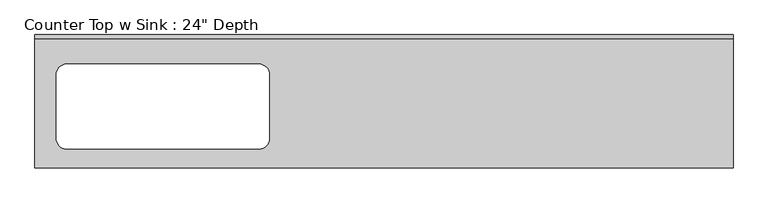
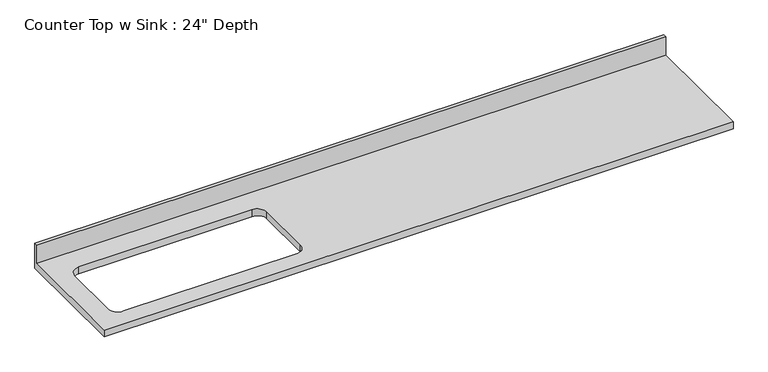
"""IFC4 building model written with IfcOpenShell, lengths in millimetres: furniture geometry."""

from ifc_helpers import new_model, si_unit, frame, origin, place, context, project, spatial, polyline, circle_curve, source, transform, mapped, element, save
from ifc_brep_helpers import plane_surface, revolved_surface, advanced_brep


def furniture_c9b163cf(model_context):
    return source(origin(), model_context, "Body", "AdvancedBrep", [
        advanced_brep(
        [(-1200.4622951, -635.0, 914.4), (2126.9377049, -635.0, 914.4), (2126.9377049, -19.05, 914.4), (-1200.4622951, -19.05, 914.4), (-1048.0622951, -139.7, 914.4), (-133.6622951, -139.7, 914.4), (-82.8622951, -190.5, 914.4), (-82.8622951, -495.3, 914.4), (-133.6622951, -546.1, 914.4), (-1048.0622951, -546.1, 914.4), (-1098.8622951, -495.3, 914.4), (-1098.8622951, -190.5, 914.4), (2126.9377049, 0.0, 876.3), (2126.9377049, -635.0, 876.3), (-1200.4622951, -635.0, 876.3), (-1200.4622951, 0.0, 876.3), (-133.6622951, -139.7, 876.3), (-1048.0622951, -139.7, 876.3), (-1098.8622951, -190.5, 876.3), (-1098.8622951, -495.3, 876.3), (-1048.0622951, -546.1, 876.3), (-133.6622951, -546.1, 876.3), (-82.8622951, -495.3, 876.3), (-82.8622951, -190.5, 876.3), (-1200.4622951, 0.0, 1016.0), (2126.9377049, 0.0, 1016.0), (-1200.4622951, -19.05, 1016.0), (2126.9377049, -19.05, 1016.0)],
        [
            (0, 1),
            (1, 2),
            (2, 3),
            (3, 0),
            (4, 5),
            (5, 6, circle_curve(frame((-133.6622951, -190.5, 914.4), z_axis=(0.0, 0.0, -1.0), x_axis=(1.0, 0.0, 0.0)), 50.8)),
            (6, 7),
            (7, 8, circle_curve(frame((-133.6622951, -495.3, 914.4), z_axis=(0.0, 0.0, -1.0), x_axis=(1.0, 0.0, 0.0)), 50.8)),
            (8, 9),
            (9, 10, circle_curve(frame((-1048.0622951, -495.3, 914.4), z_axis=(0.0, 0.0, -1.0), x_axis=(1.0, 0.0, 0.0)), 50.8)),
            (10, 11),
            (11, 4, circle_curve(frame((-1048.0622951, -190.5, 914.4), z_axis=(0.0, 0.0, -1.0), x_axis=(1.0, 0.0, 0.0)), 50.8)),
            (12, 13),
            (13, 14),
            (14, 15),
            (15, 12),
            (16, 17),
            (17, 18, circle_curve(frame((-1048.0622951, -190.5, 876.3), z_axis=(0.0, 0.0, 1.0), x_axis=(1.0, 0.0, 0.0)), 50.8)),
            (18, 19),
            (19, 20, circle_curve(frame((-1048.0622951, -495.3, 876.3), z_axis=(0.0, 0.0, 1.0), x_axis=(1.0, 0.0, 0.0)), 50.8)),
            (20, 21),
            (21, 22, circle_curve(frame((-133.6622951, -495.3, 876.3), z_axis=(0.0, 0.0, 1.0), x_axis=(1.0, 0.0, 0.0)), 50.8)),
            (22, 23),
            (23, 16, circle_curve(frame((-133.6622951, -190.5, 876.3), z_axis=(0.0, 0.0, 1.0), x_axis=(1.0, 0.0, 0.0)), 50.8)),
            (15, 24),
            (24, 25),
            (25, 12),
            (14, 0),
            (3, 26),
            (26, 24),
            (13, 1),
            (25, 27),
            (27, 2),
            (26, 27),
            (4, 17),
            (16, 5),
            (11, 18),
            (10, 19),
            (9, 20),
            (8, 21),
            (7, 22),
            (6, 23),
        ],
        [
            plane_surface(frame((-1200.4622951, 0.0, 914.4), z_axis=(0.0, 0.0, 1.0), x_axis=(-1.0, 0.0, 0.0))),
            plane_surface(frame((-1200.4622951, 0.0, 876.3), z_axis=(0.0, 0.0, -1.0), x_axis=(1.0, 0.0, 0.0))),
            plane_surface(frame((2126.9377049, 0.0, 914.4), z_axis=(0.0, 1.0, 0.0), x_axis=(0.0, 0.0, -1.0))),
            plane_surface(frame((-1200.4622951, 0.0, 914.4), z_axis=(-1.0, 0.0, 0.0), x_axis=(0.0, 0.0, -1.0))),
            plane_surface(frame((-1200.4622951, -635.0, 914.4), z_axis=(0.0, -1.0, 0.0), x_axis=(0.0, 0.0, -1.0))),
            plane_surface(frame((2126.9377049, -635.0, 914.4), z_axis=(1.0, 0.0, 0.0), x_axis=(0.0, 0.0, -1.0))),
            plane_surface(frame((-1200.4622951, 0.0, 1016.0), z_axis=(0.0, 0.0, 1.0), x_axis=(0.0, -1.0, 0.0))),
            plane_surface(frame((-1200.4622951, -19.05, 1016.0), z_axis=(0.0, -1.0, 0.0), x_axis=(0.0, 0.0, -1.0))),
            plane_surface(frame((-133.6622951, -139.7, 914.4), z_axis=(0.0, -1.0, 0.0), x_axis=(0.0, 0.0, -1.0))),
            revolved_surface(polyline([(-997.2622951000001, -190.5, 914.4), (-997.2622951000001, -190.5, 876.3)]), (-1048.0622951, -190.5, 876.3), (0.0, 0.0, 1.0)),
            plane_surface(frame((-1098.8622951, -190.5, 914.4), z_axis=(1.0, 0.0, 0.0), x_axis=(0.0, 0.0, -1.0))),
            revolved_surface(polyline([(-997.2622951000001, -495.3, 914.4), (-997.2622951000001, -495.3, 876.3)]), (-1048.0622951, -495.3, 876.3), (0.0, 0.0, 1.0)),
            plane_surface(frame((-1048.0622951, -546.1, 914.4), z_axis=(0.0, 1.0, 0.0), x_axis=(0.0, 0.0, -1.0))),
            revolved_surface(polyline([(-82.8622951, -495.3, 914.4), (-82.8622951, -495.3, 876.3)]), (-133.6622951, -495.3, 876.3), (0.0, 0.0, 1.0)),
            plane_surface(frame((-82.8622951, -495.3, 914.4), z_axis=(-1.0, 0.0, 0.0), x_axis=(0.0, 0.0, -1.0))),
            revolved_surface(polyline([(-82.8622951, -190.5, 914.4), (-82.8622951, -190.5, 876.3)]), (-133.6622951, -190.5, 876.3), (0.0, 0.0, 1.0)),
        ],
        [
            (0, [[1, 2, 3, 4], [5, 6, 7, 8, 9, 10, 11, 12]]),
            (1, [[13, 14, 15, 16], [17, 18, 19, 20, 21, 22, 23, 24]]),
            (2, [[-16, 25, 26, 27]]),
            (3, [[-15, 28, -4, 29, 30, -25]]),
            (4, [[-1, -28, -14, 31]]),
            (5, [[-13, -27, 32, 33, -2, -31]]),
            (6, [[-30, 34, -32, -26]]),
            (7, [[-34, -29, -3, -33]]),
            (8, [[35, -17, 36, -5]]),
            (9, [[-35, -12, 37, -18]]),
            (10, [[-37, -11, 38, -19]]),
            (11, [[-38, -10, 39, -20]]),
            (12, [[-39, -9, 40, -21]]),
            (13, [[-40, -8, 41, -22]]),
            (14, [[-41, -7, 42, -23]]),
            (15, [[-36, -24, -42, -6]]),
        ],
    ),
    ])


if __name__ == "__main__":
    model = new_model("IFC4")
    model_context = context("Model", 3, world=origin())
    ifc_project = project(units=[si_unit("LENGTHUNIT", "METRE", prefix="MILLI")], contexts=[model_context])
    site = spatial("IfcSite", under=ifc_project)
    building = spatial("IfcBuilding", under=site)
    placement = place(None, origin())
    furniture_shape = furniture_c9b163cf(model_context)
    element("IfcFurniture", 1, ObjectType="Counter Top w Sink : 24\" Depth", at=placement, inside=building, context=model_context, shape_type="MappedRepresentation", body=[
        mapped(furniture_shape, transform((0.0, 0.0, 0.0), x_axis=(1.0, 0.0, 0.0), y_axis=(0.0, 1.0, 0.0), z_axis=(0.0, 0.0, 1.0))),
    ])
    save(model, "model.ifc")

# Revit data of these elements
# Type "Counter Top w Sink : 24\" Depth"
#   Assembly Code = "C1030400"
#   Counter Thickness = 0' - 1 1/2"
#   Depth = 2' - 1"
#   Height = 3' - 0"
#   Length [instance default] = 8' - 0"
#   Sink Location [instance default] = 2' - 0"
#   Sink Location To Wall [instance default] = 0' - 6"
#   Sink Opening Depth [instance default] = 1' - 3"
#   Sink Opening Width [instance default] = 3' - 3"
#   Counter Top Material = none
#   Default Elevation = 0
# Element 1 (IfcFurniture, "Counter Top w Sink : 24\" Depth")
#   Length = 10' - 11"
#   Materials on its faces: "Counter Top"
# Materials
#   "Counter Top": class "Wood", colour RGB 226 177 128, transparency 0
